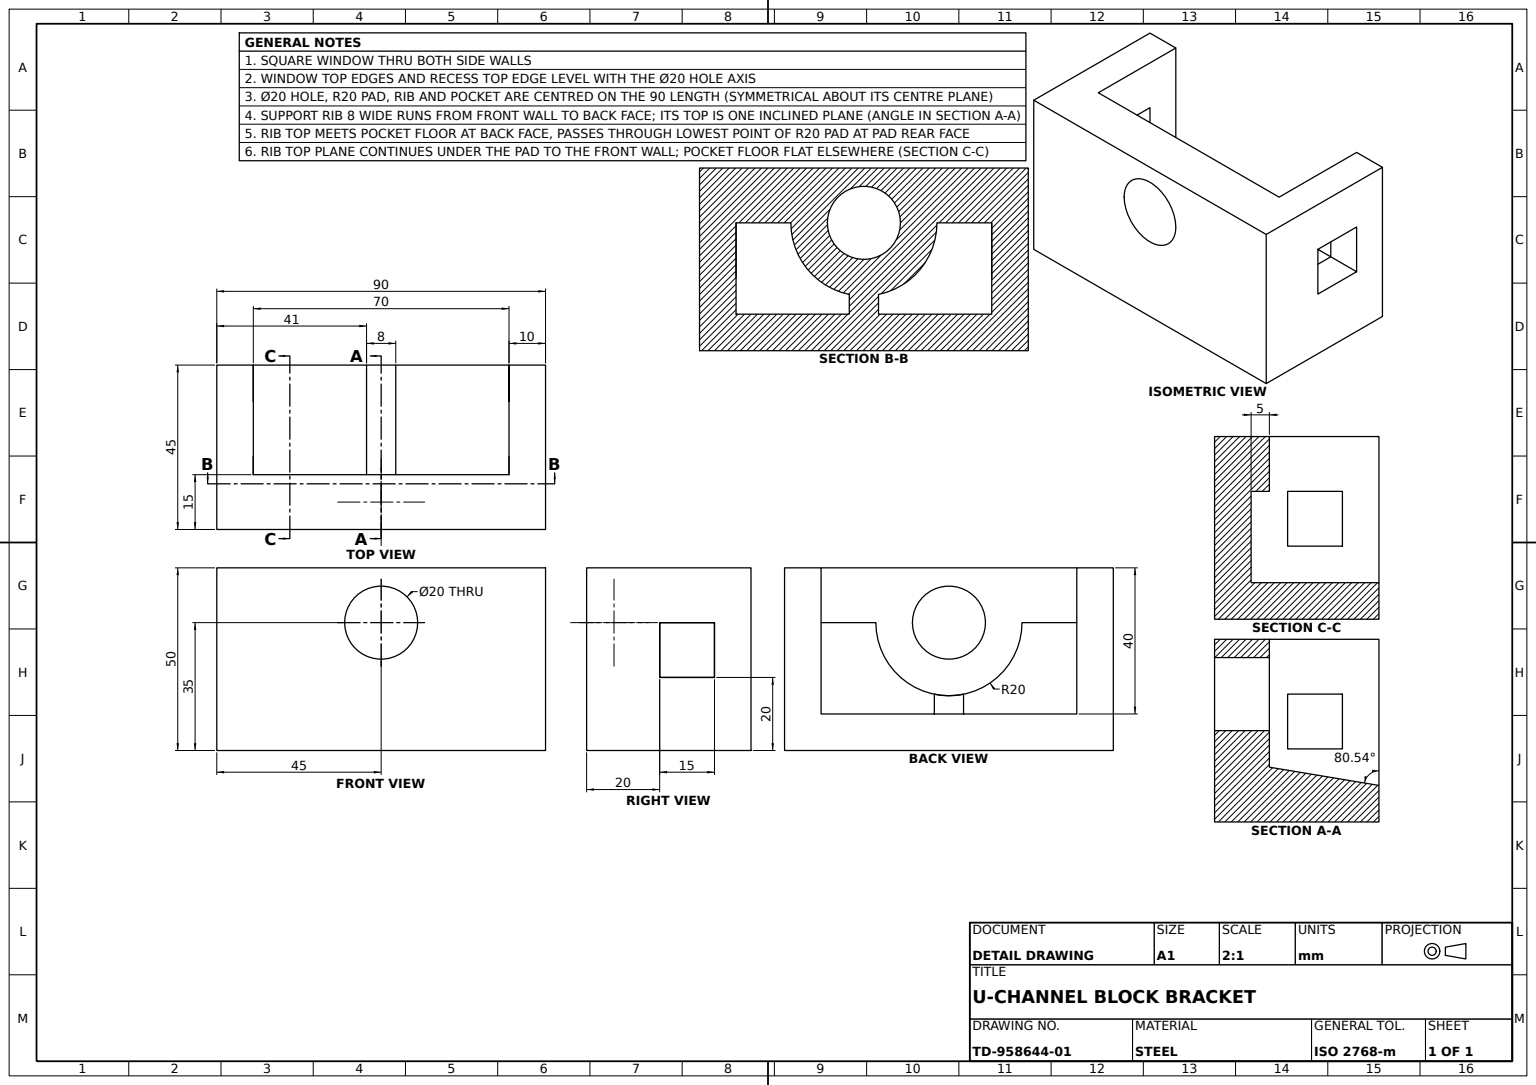
SolidWorks part; units mm, degrees
material "Plain Carbon Steel"
ref_plane "Front Plane" through (0, 0, 0) normal (0, 0, 1) x (1, 0, 0)
ref_plane "Top Plane" through (0, 0, 0) normal (0, 1, 0) x (1, 0, 0)
ref_plane "Right Plane" through (0, 0, 0) normal (1, 0, 0) x (0, 0, -1)
sketch "Block Profile Sketch" plane through (0, 0, 0) normal (1, 0, 0) x (0, 0, -1)
  line L1 (-22.5, -25) -> (22.5, -25)
  line L2 (-22.5, -25) -> (-22.5, 25)
  line L3 (-22.5, 25) -> (22.5, 25)
  line L4 (22.5, -25) -> (22.5, 25)
  line L5 (-22.5, -25) -> (22.5, 25) construction
  line L6 (-22.5, 25) -> (22.5, -25) construction
  line L7 (-2.5, -5) -> (12.5, -5)
  line L8 (-2.5, -5) -> (-2.5, 10)
  line L9 (-2.5, 10) -> (12.5, 10)
  line L10 (12.5, -5) -> (12.5, 10)
  line L11 (-2.5, -5) -> (12.5, 10) construction
  line L12 (-2.5, 10) -> (12.5, -5) construction
  point P0 (0, 0)
  point P6 (5, 2.5)
  dimension "D1" = 45
  dimension "D2" = 50
  dimension "D3" = 15
  dimension "D4" = 20
  dimension "D5" = 20
  dimension "D6" = 15
extrude "Block Body 90mm" add sketch "Block Profile Sketch" along normal mid plane 90
sketch "Center Pocket Sketch" plane through (0, 25, 0) normal (0, 1, 0) x (1, 0, 0)
  line L0 (45, 22.5) -> (-45, 22.5) construction
  line L1 (-35, 22.5) -> (35, 22.5)
  line L2 (-35, 22.5) -> (-35, -12.5)
  line L3 (-35, -12.5) -> (35, -12.5)
  line L4 (35, 22.5) -> (35, -12.5)
  point P6 (0, -12.5)
  dimension "D1" = 35
  dimension "D2" = 70
extrude "Center Pocket 35x70" cut sketch "Center Pocket Sketch" against normal blind 40
sketch "Pocket Pad Sketch" plane through (0, 0, 12.5) normal (0, 0, -1) x (-1, 0, 0)
  line L0 (35, 25) -> (-35, 25) construction
  line L1 (20, 10) -> (35, 10)
  line L2 (35, -15) -> (35, 25) construction
  line L3 (-20, 10) -> (-35, 10)
  line L4 (-35, -15) -> (-35, 25) construction
  line L5 (-35, 10) -> (-35, 25)
  line L6 (-35, -15) -> (-35, 25) construction
  line L7 (-35, 25) -> (35, 25)
  line L8 (35, 25) -> (35, 10)
  arc A0 (-20, 10) -> (20, 10) centre (0, 10) ccw
  circle A1 centre (0, 10) radius 10
  dimension "D2" = 20
  dimension "D3" = 20
  dimension "D1" = 15
extrude "Pocket Pad 5mm" add sketch "Pocket Pad Sketch" along normal blind 5
sketch "Side Hole Sketch" plane through (0, 0, 12.5) normal (0, 0, -1) x (-1, 0, 0)
  circle A0 centre (0, 10) radius 10 construction
  circle A1 centre (0, 10) radius 10
extrude "Side Hole" cut sketch "Side Hole Sketch" against normal up to next
sketch "Support Rib Sketch" plane through (0, 0, 0) normal (1, 0, 0) x (0, 0, -1)
  line L0 (-7.5, -10) -> (22.5, -15)
rib "Support Rib 8mm" sketch "Support Rib Sketch" sketch "Support Rib Sketch" thickness 8 extrusion direction parallel to sketch draft on no parameters "D1"=8
